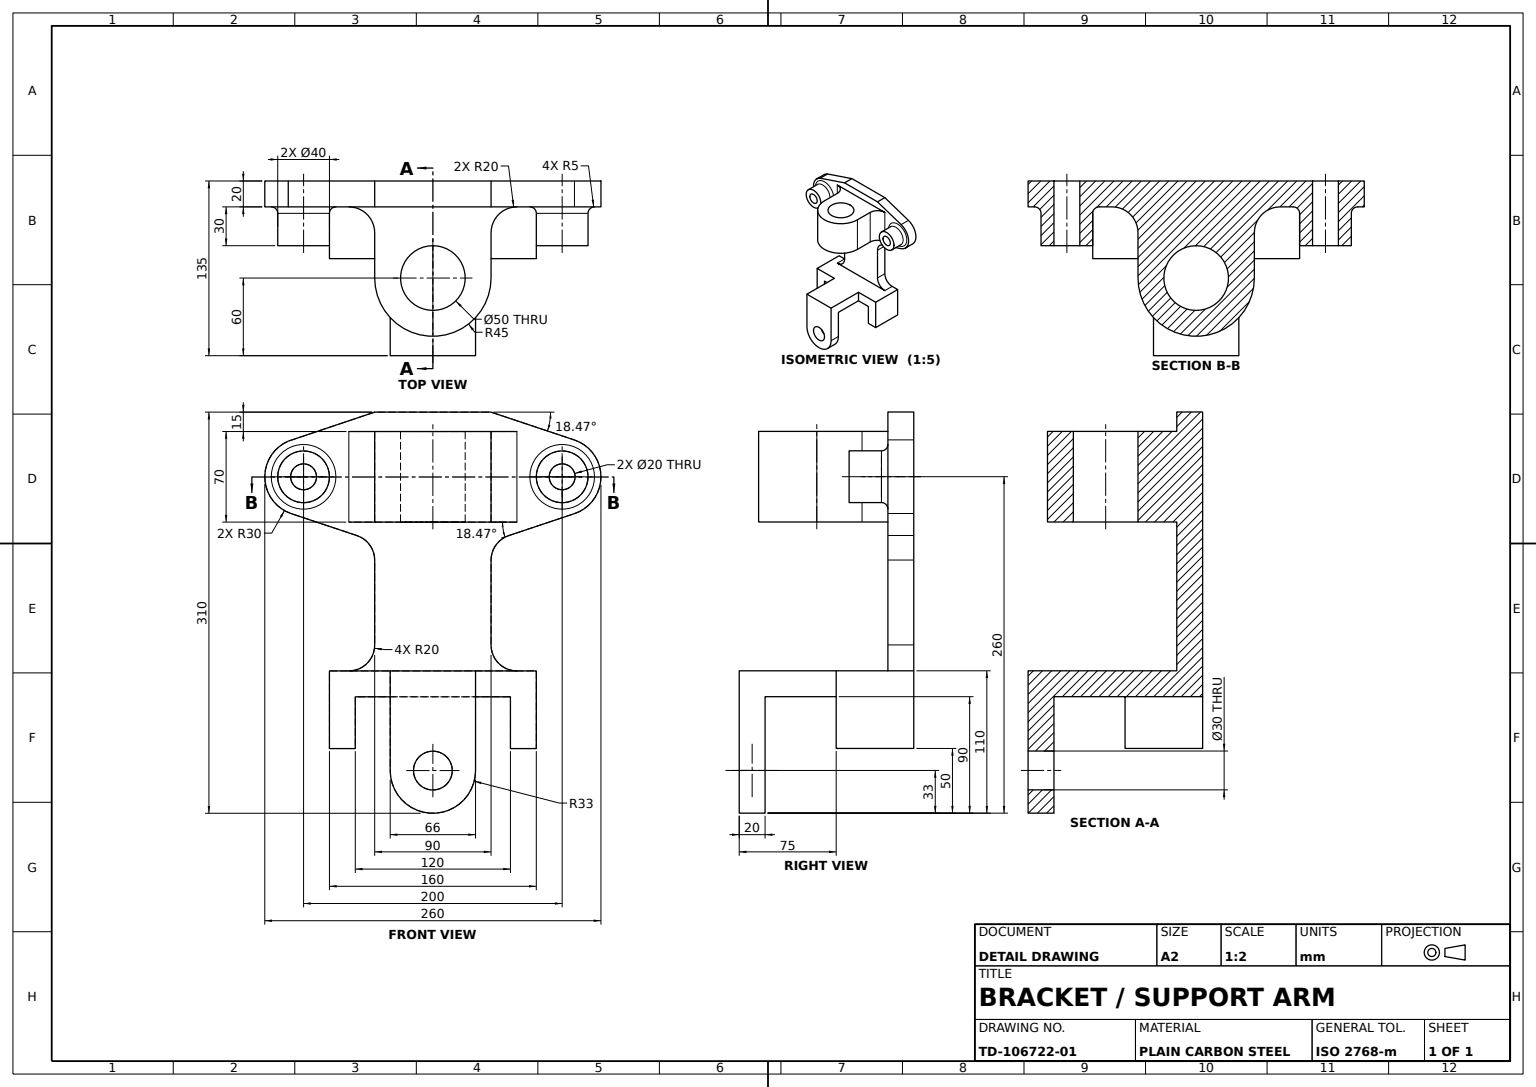
from build123d import *

# Parameters (mm, degrees)
BASE_BLOCK_DEPTH               = 60
CLEVIS_LUG_DEPTH               = 20
LUG_EXTENSION_DEPTH            = 20
PIN_HOLE_SKETCH_30_R           = 15
CLEVIS_PIN_HOLE_30_DEPTH       = 215
UPRIGHT_WEB_DEPTH              = 20
FLANGE_PLATE_DEPTH             = 20
WEB_FLANGE_FILLET_R20_A_R      = 20
WEB_FLANGE_FILLET_R20_B_R      = 20
WEB_BASE_FILLET_R20_A_R        = 20
WEB_BASE_FILLET_R20_B_R        = 20
HUB_BOSS_DEPTH                 = 35
HUB_WEB_FILLET_R20_A_R         = 20
HUB_WEB_FILLET_R20_B_R         = 20
MOUNTING_BOSSES_SKETCH_2X_40_R = 20
MOUNTING_BOSSES_2X_40_DEPTH    = 30
MOUNTING_BOSS_FILLET_R5_A_R    = 5
MOUNTING_BOSS_FILLET_R5_B_R    = 5
HUB_BORE_SKETCH_50_R           = 25
HUB_BORE_50_DEPTH              = 82
MOUNTING_HOLES_SKETCH_2X_20_R  = 10
MOUNTING_HOLES_2X_20_DEPTH     = 82


with BuildPart() as part:
    # Base Profile Sketch → Base Block (new body)
    with BuildSketch(Plane.XY):
        Polygon((60, 0), (80, 0), (80, 60), (-80, 60), (-80, 0), (-60, 0), (-60, 40), (60, 40), align=None)
    extrude(amount=BASE_BLOCK_DEPTH)

    # Clevis Lug Sketch → Clevis Lug (add)
    with BuildSketch(Plane(origin=(0, 60, 0), x_dir=(1, 0, 0), z_dir=(0, 1, 0))):
        Polygon((0, -135), (33, -135), (33, -60), (-33, -60), (-33, -135), align=None)
    extrude(amount=-CLEVIS_LUG_DEPTH)

    # Lug Extension Sketch → Lug Extension (add)
    with BuildSketch(Plane.XY.offset(135)):
        with BuildLine():
            Line((33, -17), (33, 40))
            Line((33, 40), (-33, 40))
            Line((-33, 40), (-33, -17))
            ThreePointArc((-33, -17), (0, -50), (33, -17))
        make_face()
    extrude(amount=-LUG_EXTENSION_DEPTH)

    # Pin Hole Sketch Ø30 → Clevis Pin Hole Ø30 (cut)
    with BuildSketch(Plane.XY.offset(135)):
        with Locations((0, -17)):
            Circle(PIN_HOLE_SKETCH_30_R)
    extrude(amount=-CLEVIS_PIN_HOLE_30_DEPTH, mode=Mode.SUBTRACT)

    # Upright Web Sketch → Upright Web (add)
    with BuildSketch(Plane(origin=(0, 0, 0), x_dir=(-1, 0, 0), z_dir=(0, 0, -1))):
        Polygon((0, 60), (45, 60), (45, 160), (-45, 160), (-45, 60), align=None)
    extrude(amount=-UPRIGHT_WEB_DEPTH)

    # Flange Plate Sketch → Flange Plate (add)
    with BuildSketch(Plane.XY.offset(20)):
        with BuildLine():
            Line((0, 260), (45, 260))
            Line((45, 260), (109.504258609, 238.45468447))
            ThreePointArc((109.504258609, 238.45468447), (130, 210), (109.504258609, 181.54531553))
            Line((109.504258609, 181.54531553), (45, 160))
            Line((45, 160), (-45, 160))
            Line((-45, 160), (-109.504258609, 181.54531553))
            ThreePointArc((-109.504258609, 181.54531553), (-129.973433228, 208.737739921), (-111.86296755, 237.554854398))
            Line((-111.86296755, 237.554854398), (-45, 260))
            Line((-45, 260), (0, 260))
        make_face()
    extrude(amount=-FLANGE_PLATE_DEPTH)

    # Web-Flange Fillet R20 A
    web_flange_fillet_r20_a_edges = [part.edges().sort_by_distance(p)[0] for p in [
        (-45, 160, 10),
    ]]
    fillet(web_flange_fillet_r20_a_edges, radius=WEB_FLANGE_FILLET_R20_A_R)

    # Web-Flange Fillet R20 B
    web_flange_fillet_r20_b_edges = [part.edges().sort_by_distance(p)[0] for p in [
        (45, 160, 10),
    ]]
    fillet(web_flange_fillet_r20_b_edges, radius=WEB_FLANGE_FILLET_R20_B_R)

    # Web-Base Fillet R20 A
    web_base_fillet_r20_a_edges = [part.edges().sort_by_distance(p)[0] for p in [
        (45, 60, 10),
    ]]
    fillet(web_base_fillet_r20_a_edges, radius=WEB_BASE_FILLET_R20_A_R)

    # Web-Base Fillet R20 B
    web_base_fillet_r20_b_edges = [part.edges().sort_by_distance(p)[0] for p in [
        (-45, 60, 10),
    ]]
    fillet(web_base_fillet_r20_b_edges, radius=WEB_BASE_FILLET_R20_B_R)

    # Hub Sketch → Hub Boss (add, symmetric)
    with BuildSketch(Plane(origin=(0, 210, 0), x_dir=(1, 0, 0), z_dir=(0, 1, 0))):
        with BuildLine():
            Line((-45, -75), (-45, -20))
            Line((-45, -20), (45, -20))
            Line((45, -20), (45, -75))
            ThreePointArc((45, -75), (0, -120), (-45, -75))
        make_face()
    extrude(amount=HUB_BOSS_DEPTH, both=True)

    # Hub-Web Fillet R20 A
    hub_web_fillet_r20_a_edges = [part.edges().sort_by_distance(p)[0] for p in [
        (-45, 210, 20),
    ]]
    fillet(hub_web_fillet_r20_a_edges, radius=HUB_WEB_FILLET_R20_A_R)

    # Hub-Web Fillet R20 B
    hub_web_fillet_r20_b_edges = [part.edges().sort_by_distance(p)[0] for p in [
        (45, 210, 20),
    ]]
    fillet(hub_web_fillet_r20_b_edges, radius=HUB_WEB_FILLET_R20_B_R)

    # Mounting Bosses Sketch 2xØ40 → Mounting Bosses 2xØ40 (add)
    with BuildSketch(Plane.XY.offset(20)):
        with Locations(Location((100, 210, 0), (0, 0, 180))):
            Circle(MOUNTING_BOSSES_SKETCH_2X_40_R)
        with Locations(Location((-100, 210, 0), (0, 0, 180))):
            Circle(MOUNTING_BOSSES_SKETCH_2X_40_R)
    extrude(amount=MOUNTING_BOSSES_2X_40_DEPTH)

    # Mounting Boss Fillet R5 A
    mounting_boss_fillet_r5_a_edges = [part.edges().sort_by_distance(p)[0] for p in [
        (120, 210, 20),
    ]]
    fillet(mounting_boss_fillet_r5_a_edges, radius=MOUNTING_BOSS_FILLET_R5_A_R)

    # Mounting Boss Fillet R5 B
    mounting_boss_fillet_r5_b_edges = [part.edges().sort_by_distance(p)[0] for p in [
        (-80, 210, 20),
    ]]
    fillet(mounting_boss_fillet_r5_b_edges, radius=MOUNTING_BOSS_FILLET_R5_B_R)

    # Hub Bore Sketch Ø50 → Hub Bore Ø50 (cut)
    with BuildSketch(Plane(origin=(0, 245, 0), x_dir=(1, 0, 0), z_dir=(0, 1, 0))):
        with Locations(Location((0, -75, 0), (0, 0, 270))):
            Circle(HUB_BORE_SKETCH_50_R)
    extrude(amount=-HUB_BORE_50_DEPTH, mode=Mode.SUBTRACT)

    # Mounting Holes Sketch 2xØ20 → Mounting Holes 2xØ20 (cut)
    with BuildSketch(Plane.XY.offset(50)):
        with Locations((100, 210)):
            Circle(MOUNTING_HOLES_SKETCH_2X_20_R)
        with Locations((-100, 210)):
            Circle(MOUNTING_HOLES_SKETCH_2X_20_R)
    extrude(amount=-MOUNTING_HOLES_2X_20_DEPTH, mode=Mode.SUBTRACT)


solid = part.part
